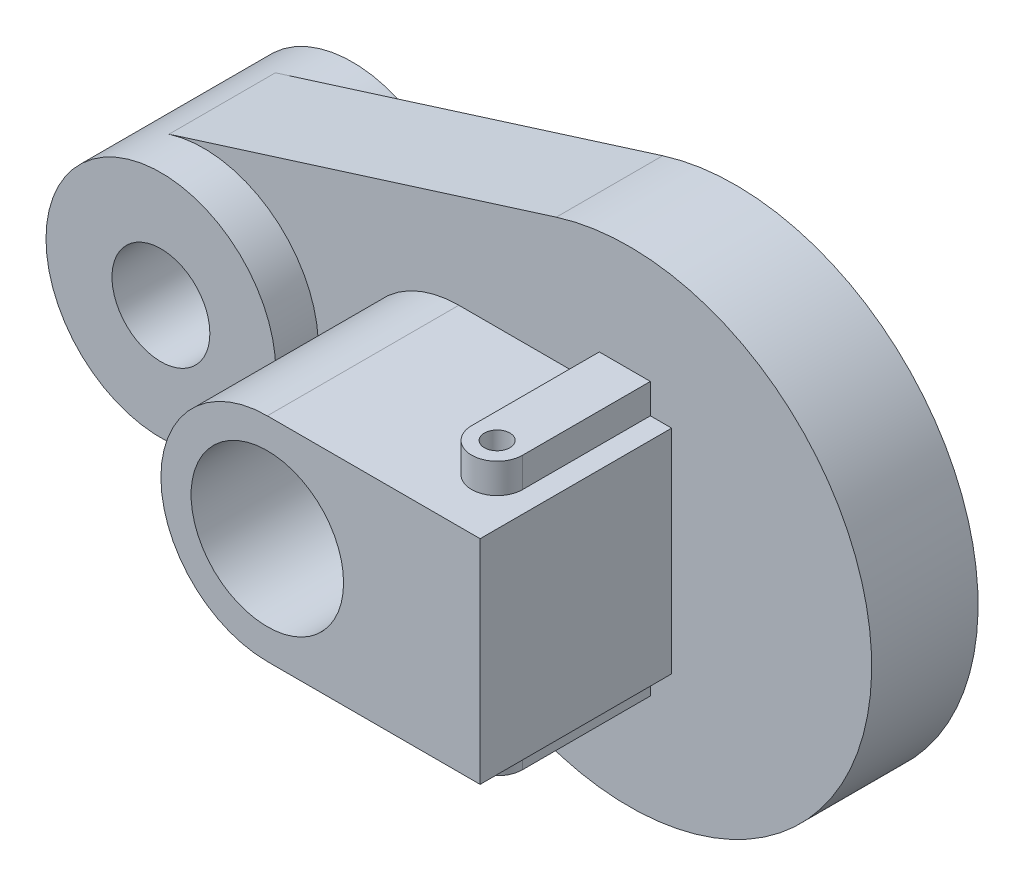
ISO-10303-21;
HEADER;
FILE_DESCRIPTION(('STEP AP214'),'2;1');
FILE_NAME('part.step','',(''),(''),'','','');
FILE_SCHEMA(('AUTOMOTIVE_DESIGN { 1 0 10303 214 1 1 1 1 }'));
ENDSEC;
DATA;
#1=APPLICATION_CONTEXT('core data for automotive mechanical design processes');
#2=APPLICATION_PROTOCOL_DEFINITION('international standard','automotive_design',2000,#1);
#3=PRODUCT_CONTEXT('',#1,'mechanical');
#4=PRODUCT('Part','Part','',(#3));
#5=PRODUCT_RELATED_PRODUCT_CATEGORY('part','',(#4));
#6=PRODUCT_DEFINITION_FORMATION('','',#4);
#7=PRODUCT_DEFINITION_CONTEXT('part definition',#1,'design');
#8=PRODUCT_DEFINITION('design','',#6,#7);
#9=PRODUCT_DEFINITION_SHAPE('','',#8);
#10=(LENGTH_UNIT() NAMED_UNIT(*) SI_UNIT(.MILLI.,.METRE.));
#11=(NAMED_UNIT(*) PLANE_ANGLE_UNIT() SI_UNIT($,.RADIAN.));
#12=(NAMED_UNIT(*) SI_UNIT($,.STERADIAN.) SOLID_ANGLE_UNIT());
#13=UNCERTAINTY_MEASURE_WITH_UNIT(LENGTH_MEASURE(1.E-05),#10,'distance_accuracy_value','');
#14=(GEOMETRIC_REPRESENTATION_CONTEXT(3) GLOBAL_UNCERTAINTY_ASSIGNED_CONTEXT((#13)) GLOBAL_UNIT_ASSIGNED_CONTEXT((#10,
#11,#12)) REPRESENTATION_CONTEXT('',''));
#15=CARTESIAN_POINT('',(0.,0.,0.));
#16=DIRECTION('',(0.,0.,1.));
#17=DIRECTION('',(1.,0.,0.));
#18=AXIS2_PLACEMENT_3D('',#15,#16,#17);
#19=CARTESIAN_POINT('',(0.,0.,25.));
#20=DIRECTION('',(0.,0.,1.));
#21=DIRECTION('',(1.,0.,0.));
#22=AXIS2_PLACEMENT_3D('',#19,#20,#21);
#23=PLANE('',#22);
#24=CARTESIAN_POINT('',(-99.9999999999951,0.,25.));
#25=DIRECTION('',(0.,0.,1.));
#26=DIRECTION('',(1.,0.,0.));
#27=AXIS2_PLACEMENT_3D('',#24,#25,#26);
#28=CIRCLE('',#27,26.9999999999953);
#29=CARTESIAN_POINT('',(-108.050824082347,-25.7717719917503,25.));
#30=VERTEX_POINT('',#29);
#31=CARTESIAN_POINT('',(-108.100000000003,25.7563584382502,25.));
#32=VERTEX_POINT('',#31);
#33=EDGE_CURVE('E11',#30,#32,#28,.T.);
#34=ORIENTED_EDGE('',*,*,#33,.F.);
#35=DIRECTION('',(0.954225072155131,-0.299089471012498,0.));
#36=VECTOR('',#35,1.);
#37=CARTESIAN_POINT('',(-17.0208632069058,-54.3039324211904,25.));
#38=LINE('',#37,#36);
#39=CARTESIAN_POINT('',(-20.0941700871881,-53.3406442453654,25.));
#40=VERTEX_POINT('',#39);
#41=EDGE_CURVE('E329',#30,#40,#38,.T.);
#42=ORIENTED_EDGE('',*,*,#41,.T.);
#43=CARTESIAN_POINT('',(0.,0.,25.));
#44=DIRECTION('',(0.,0.,1.));
#45=DIRECTION('',(1.,0.,0.));
#46=AXIS2_PLACEMENT_3D('',#43,#44,#45);
#47=CIRCLE('',#46,57.0000000000306);
#48=CARTESIAN_POINT('',(-17.1000000000286,54.3745344807889,25.));
#49=VERTEX_POINT('',#48);
#50=EDGE_CURVE('E338',#40,#49,#47,.T.);
#51=ORIENTED_EDGE('',*,*,#50,.T.);
#52=DIRECTION('',(0.953939201416839,0.30000000000034,0.));
#53=VECTOR('',#52,1.);
#54=CARTESIAN_POINT('',(-17.1000000000286,54.3745344807889,25.));
#55=LINE('',#54,#53);
#56=EDGE_CURVE('E343',#32,#49,#55,.T.);
#57=ORIENTED_EDGE('',*,*,#56,.F.);
#58=EDGE_LOOP('',(#34,#42,#51,#57));
#59=FACE_BOUND('',#58,.T.);
#60=DIRECTION('',(-1.,0.,0.));
#61=VECTOR('',#60,1.);
#62=CARTESIAN_POINT('',(-40.,25.,25.));
#63=LINE('',#62,#61);
#64=CARTESIAN_POINT('',(-6.99999999999999,25.,25.));
#65=VERTEX_POINT('',#64);
#66=CARTESIAN_POINT('',(-40.,25.,25.));
#67=VERTEX_POINT('',#66);
#68=EDGE_CURVE('E257',#65,#67,#63,.T.);
#69=ORIENTED_EDGE('',*,*,#68,.F.);
#70=DIRECTION('',(0.,-1.,0.));
#71=VECTOR('',#70,1.);
#72=CARTESIAN_POINT('',(-6.99999999999999,32.,25.));
#73=LINE('',#72,#71);
#74=CARTESIAN_POINT('',(-6.99999999999999,32.,25.));
#75=VERTEX_POINT('',#74);
#76=EDGE_CURVE('E63',#75,#65,#73,.T.);
#77=ORIENTED_EDGE('',*,*,#76,.F.);
#78=DIRECTION('',(-1.,0.,0.));
#79=VECTOR('',#78,1.);
#80=CARTESIAN_POINT('',(-6.99999999999999,32.,25.));
#81=LINE('',#80,#79);
#82=CARTESIAN_POINT('',(5.00000000000001,32.,25.));
#83=VERTEX_POINT('',#82);
#84=EDGE_CURVE('E68',#83,#75,#81,.T.);
#85=ORIENTED_EDGE('',*,*,#84,.F.);
#86=DIRECTION('',(0.,-1.,0.));
#87=VECTOR('',#86,1.);
#88=CARTESIAN_POINT('',(5.00000000000001,32.,25.));
#89=LINE('',#88,#87);
#90=CARTESIAN_POINT('',(5.00000000000001,25.,25.));
#91=VERTEX_POINT('',#90);
#92=EDGE_CURVE('E186',#83,#91,#89,.T.);
#93=ORIENTED_EDGE('',*,*,#92,.T.);
#94=CARTESIAN_POINT('',(10.,25.,25.));
#95=VERTEX_POINT('',#94);
#96=EDGE_CURVE('E244',#95,#91,#63,.T.);
#97=ORIENTED_EDGE('',*,*,#96,.F.);
#98=DIRECTION('',(0.,1.,0.));
#99=VECTOR('',#98,1.);
#100=CARTESIAN_POINT('',(10.,25.,25.));
#101=LINE('',#100,#99);
#102=CARTESIAN_POINT('',(10.,-25.,25.));
#103=VERTEX_POINT('',#102);
#104=EDGE_CURVE('E256',#103,#95,#101,.T.);
#105=ORIENTED_EDGE('',*,*,#104,.F.);
#106=DIRECTION('',(1.,0.,0.));
#107=VECTOR('',#106,1.);
#108=CARTESIAN_POINT('',(10.,-25.,25.));
#109=LINE('',#108,#107);
#110=CARTESIAN_POINT('',(5.00000000000001,-25.,25.));
#111=VERTEX_POINT('',#110);
#112=EDGE_CURVE('E251',#111,#103,#109,.T.);
#113=ORIENTED_EDGE('',*,*,#112,.F.);
#114=DIRECTION('',(0.,1.,0.));
#115=VECTOR('',#114,1.);
#116=CARTESIAN_POINT('',(5.00000000000001,-32.,25.));
#117=LINE('',#116,#115);
#118=CARTESIAN_POINT('',(5.00000000000001,-32.,25.));
#119=VERTEX_POINT('',#118);
#120=EDGE_CURVE('E233',#119,#111,#117,.T.);
#121=ORIENTED_EDGE('',*,*,#120,.F.);
#122=DIRECTION('',(1.,0.,0.));
#123=VECTOR('',#122,1.);
#124=CARTESIAN_POINT('',(-6.99999999999999,-32.,25.));
#125=LINE('',#124,#123);
#126=CARTESIAN_POINT('',(-6.99999999999999,-32.,25.));
#127=VERTEX_POINT('',#126);
#128=EDGE_CURVE('E203',#127,#119,#125,.T.);
#129=ORIENTED_EDGE('',*,*,#128,.F.);
#130=DIRECTION('',(0.,1.,0.));
#131=VECTOR('',#130,1.);
#132=CARTESIAN_POINT('',(-6.99999999999999,-32.,25.));
#133=LINE('',#132,#131);
#134=CARTESIAN_POINT('',(-6.99999999999999,-25.,25.));
#135=VERTEX_POINT('',#134);
#136=EDGE_CURVE('E212',#127,#135,#133,.T.);
#137=ORIENTED_EDGE('',*,*,#136,.T.);
#138=CARTESIAN_POINT('',(-40.,-25.,25.));
#139=VERTEX_POINT('',#138);
#140=EDGE_CURVE('E253',#139,#135,#109,.T.);
#141=ORIENTED_EDGE('',*,*,#140,.F.);
#142=CARTESIAN_POINT('',(-40.,0.,25.));
#143=DIRECTION('',(0.,0.,1.));
#144=DIRECTION('',(1.,0.,0.));
#145=AXIS2_PLACEMENT_3D('',#142,#143,#144);
#146=CIRCLE('',#145,25.);
#147=EDGE_CURVE('E238',#67,#139,#146,.T.);
#148=ORIENTED_EDGE('',*,*,#147,.F.);
#149=EDGE_LOOP('',(#69,#77,#85,#93,#97,#105,#113,#121,#129,#137,#141,#148));
#150=FACE_BOUND('',#149,.T.);
#151=ADVANCED_FACE('F50',(#59,#150),#23,.T.);
#152=CARTESIAN_POINT('',(-40.,25.,70.));
#153=DIRECTION('',(0.,-1.,0.));
#154=DIRECTION('',(0.,0.,-1.));
#155=AXIS2_PLACEMENT_3D('',#152,#153,#154);
#156=PLANE('',#155);
#157=DIRECTION('',(0.,0.,1.));
#158=VECTOR('',#157,1.);
#159=CARTESIAN_POINT('',(-6.99999999999999,25.,55.));
#160=LINE('',#159,#158);
#161=CARTESIAN_POINT('',(-6.99999999999999,25.,55.));
#162=VERTEX_POINT('',#161);
#163=EDGE_CURVE('E177',#65,#162,#160,.T.);
#164=ORIENTED_EDGE('',*,*,#163,.F.);
#165=ORIENTED_EDGE('',*,*,#68,.T.);
#166=DIRECTION('',(0.,0.,-1.));
#167=VECTOR('',#166,1.);
#168=CARTESIAN_POINT('',(-40.,25.,70.));
#169=LINE('',#168,#167);
#170=CARTESIAN_POINT('',(-40.,25.,70.));
#171=VERTEX_POINT('',#170);
#172=EDGE_CURVE('E252',#171,#67,#169,.T.);
#173=ORIENTED_EDGE('',*,*,#172,.F.);
#174=DIRECTION('',(-1.,0.,0.));
#175=VECTOR('',#174,1.);
#176=CARTESIAN_POINT('',(-40.,25.,70.));
#177=LINE('',#176,#175);
#178=CARTESIAN_POINT('',(10.,25.,70.));
#179=VERTEX_POINT('',#178);
#180=EDGE_CURVE('E248',#179,#171,#177,.T.);
#181=ORIENTED_EDGE('',*,*,#180,.F.);
#182=DIRECTION('',(0.,0.,-1.));
#183=VECTOR('',#182,1.);
#184=CARTESIAN_POINT('',(10.,25.,70.));
#185=LINE('',#184,#183);
#186=EDGE_CURVE('E263',#179,#95,#185,.T.);
#187=ORIENTED_EDGE('',*,*,#186,.T.);
#188=ORIENTED_EDGE('',*,*,#96,.T.);
#189=DIRECTION('',(0.,0.,-1.));
#190=VECTOR('',#189,1.);
#191=CARTESIAN_POINT('',(5.00000000000001,25.,25.));
#192=LINE('',#191,#190);
#193=CARTESIAN_POINT('',(5.00000000000001,25.,55.));
#194=VERTEX_POINT('',#193);
#195=EDGE_CURVE('E200',#194,#91,#192,.T.);
#196=ORIENTED_EDGE('',*,*,#195,.F.);
#197=CARTESIAN_POINT('',(-0.999999999999991,25.,55.));
#198=DIRECTION('',(0.,1.,0.));
#199=DIRECTION('',(0.,0.,1.));
#200=AXIS2_PLACEMENT_3D('',#197,#198,#199);
#201=CIRCLE('',#200,6.);
#202=EDGE_CURVE('E193',#162,#194,#201,.T.);
#203=ORIENTED_EDGE('',*,*,#202,.F.);
#204=EDGE_LOOP('',(#164,#165,#173,#181,#187,#188,#196,#203));
#205=FACE_BOUND('',#204,.T.);
#206=ADVANCED_FACE('F374',(#205),#156,.F.);
#207=CARTESIAN_POINT('',(10.,-25.,70.));
#208=DIRECTION('',(0.,1.,0.));
#209=DIRECTION('',(0.,0.,1.));
#210=AXIS2_PLACEMENT_3D('',#207,#208,#209);
#211=PLANE('',#210);
#212=DIRECTION('',(0.,0.,1.));
#213=VECTOR('',#212,1.);
#214=CARTESIAN_POINT('',(5.00000000000001,-25.,25.));
#215=LINE('',#214,#213);
#216=CARTESIAN_POINT('',(5.00000000000001,-25.,55.));
#217=VERTEX_POINT('',#216);
#218=EDGE_CURVE('E205',#111,#217,#215,.T.);
#219=ORIENTED_EDGE('',*,*,#218,.F.);
#220=ORIENTED_EDGE('',*,*,#112,.T.);
#221=DIRECTION('',(0.,0.,-1.));
#222=VECTOR('',#221,1.);
#223=CARTESIAN_POINT('',(10.,-25.,70.));
#224=LINE('',#223,#222);
#225=CARTESIAN_POINT('',(10.,-25.,70.));
#226=VERTEX_POINT('',#225);
#227=EDGE_CURVE('E269',#226,#103,#224,.T.);
#228=ORIENTED_EDGE('',*,*,#227,.F.);
#229=DIRECTION('',(1.,0.,0.));
#230=VECTOR('',#229,1.);
#231=CARTESIAN_POINT('',(10.,-25.,70.));
#232=LINE('',#231,#230);
#233=CARTESIAN_POINT('',(-40.,-25.,70.));
#234=VERTEX_POINT('',#233);
#235=EDGE_CURVE('E242',#234,#226,#232,.T.);
#236=ORIENTED_EDGE('',*,*,#235,.F.);
#237=DIRECTION('',(0.,0.,-1.));
#238=VECTOR('',#237,1.);
#239=CARTESIAN_POINT('',(-40.,-25.,70.));
#240=LINE('',#239,#238);
#241=EDGE_CURVE('E268',#234,#139,#240,.T.);
#242=ORIENTED_EDGE('',*,*,#241,.T.);
#243=ORIENTED_EDGE('',*,*,#140,.T.);
#244=DIRECTION('',(0.,0.,-1.));
#245=VECTOR('',#244,1.);
#246=CARTESIAN_POINT('',(-6.99999999999999,-25.,55.));
#247=LINE('',#246,#245);
#248=CARTESIAN_POINT('',(-6.99999999999999,-25.,55.));
#249=VERTEX_POINT('',#248);
#250=EDGE_CURVE('E206',#249,#135,#247,.T.);
#251=ORIENTED_EDGE('',*,*,#250,.F.);
#252=CARTESIAN_POINT('',(-0.999999999999989,-25.,55.));
#253=DIRECTION('',(0.,-1.,0.));
#254=DIRECTION('',(0.,0.,-1.));
#255=AXIS2_PLACEMENT_3D('',#252,#253,#254);
#256=CIRCLE('',#255,6.);
#257=EDGE_CURVE('E217',#217,#249,#256,.T.);
#258=ORIENTED_EDGE('',*,*,#257,.F.);
#259=EDGE_LOOP('',(#219,#220,#228,#236,#242,#243,#251,#258));
#260=FACE_BOUND('',#259,.T.);
#261=ADVANCED_FACE('F367',(#260),#211,.F.);
#262=CARTESIAN_POINT('',(0.,0.,0.));
#263=DIRECTION('',(0.,0.,1.));
#264=DIRECTION('',(1.,0.,0.));
#265=AXIS2_PLACEMENT_3D('',#262,#263,#264);
#266=PLANE('',#265);
#267=CARTESIAN_POINT('',(-99.9999999999951,0.,0.));
#268=DIRECTION('',(0.,0.,-1.));
#269=DIRECTION('',(-1.,0.,0.));
#270=AXIS2_PLACEMENT_3D('',#267,#268,#269);
#271=CIRCLE('',#270,27.0000000000047);
#272=CARTESIAN_POINT('',(-108.100000000006,25.7563584382591,0.));
#273=VERTEX_POINT('',#272);
#274=CARTESIAN_POINT('',(-108.050824073021,-25.7717719946737,0.));
#275=VERTEX_POINT('',#274);
#276=EDGE_CURVE('E280',#273,#275,#271,.T.);
#277=ORIENTED_EDGE('',*,*,#276,.F.);
#278=DIRECTION('',(0.953939201416839,0.30000000000034,0.));
#279=VECTOR('',#278,1.);
#280=CARTESIAN_POINT('',(-17.1000000000286,54.3745344807889,0.));
#281=LINE('',#280,#279);
#282=CARTESIAN_POINT('',(-17.1000000000286,54.3745344807889,0.));
#283=VERTEX_POINT('',#282);
#284=EDGE_CURVE('E342',#273,#283,#281,.T.);
#285=ORIENTED_EDGE('',*,*,#284,.T.);
#286=CARTESIAN_POINT('',(0.,0.,0.));
#287=DIRECTION('',(0.,0.,1.));
#288=DIRECTION('',(1.,0.,0.));
#289=AXIS2_PLACEMENT_3D('',#286,#287,#288);
#290=CIRCLE('',#289,57.0000000000306);
#291=CARTESIAN_POINT('',(-20.0941700871881,-53.3406442453654,0.));
#292=VERTEX_POINT('',#291);
#293=EDGE_CURVE('E344',#292,#283,#290,.T.);
#294=ORIENTED_EDGE('',*,*,#293,.F.);
#295=DIRECTION('',(0.954225072155131,-0.299089471012498,0.));
#296=VECTOR('',#295,1.);
#297=CARTESIAN_POINT('',(-17.0208632069058,-54.3039324211904,0.));
#298=LINE('',#297,#296);
#299=EDGE_CURVE('E300',#275,#292,#298,.T.);
#300=ORIENTED_EDGE('',*,*,#299,.F.);
#301=EDGE_LOOP('',(#277,#285,#294,#300));
#302=FACE_BOUND('',#301,.T.);
#303=ADVANCED_FACE('F370',(#302),#266,.F.);
#304=CARTESIAN_POINT('',(-17.1000000000286,54.3745344807889,25.));
#305=DIRECTION('',(-0.30000000000034,0.953939201416839,0.));
#306=DIRECTION('',(-0.953939201416839,-0.30000000000034,0.));
#307=AXIS2_PLACEMENT_3D('',#304,#305,#306);
#308=PLANE('',#307);
#309=ORIENTED_EDGE('',*,*,#284,.F.);
#310=DIRECTION('',(0.,0.,-1.));
#311=VECTOR('',#310,1.);
#312=CARTESIAN_POINT('',(-108.100000000004,25.7563584382527,25.));
#313=LINE('',#312,#311);
#314=EDGE_CURVE('E57',#32,#273,#313,.T.);
#315=ORIENTED_EDGE('',*,*,#314,.F.);
#316=ORIENTED_EDGE('',*,*,#56,.T.);
#317=DIRECTION('',(0.,0.,-1.));
#318=VECTOR('',#317,1.);
#319=CARTESIAN_POINT('',(-17.1000000000286,54.3745344807889,25.));
#320=LINE('',#319,#318);
#321=EDGE_CURVE('E336',#49,#283,#320,.T.);
#322=ORIENTED_EDGE('',*,*,#321,.T.);
#323=EDGE_LOOP('',(#309,#315,#316,#322));
#324=FACE_BOUND('',#323,.T.);
#325=ADVANCED_FACE('F47',(#324),#308,.T.);
#326=CARTESIAN_POINT('',(-99.9999999999951,0.,25.));
#327=DIRECTION('',(0.,0.,-1.));
#328=DIRECTION('',(-1.,0.,0.));
#329=AXIS2_PLACEMENT_3D('',#326,#327,#328);
#330=CYLINDRICAL_SURFACE('',#329,26.999999999998);
#331=ORIENTED_EDGE('',*,*,#314,.T.);
#332=ORIENTED_EDGE('',*,*,#276,.T.);
#333=CARTESIAN_POINT('',(-108.100000000004,-25.7563584382527,0.));
#334=DIRECTION('',(0.95422507215511,-0.299089471012563,0.));
#335=VECTOR('',#334,1.);
#336=LINE('',#333,#335);
#337=CARTESIAN_POINT('',(-108.100000000004,-25.7563584382527,0.));
#338=VERTEX_POINT('',#337);
#339=EDGE_CURVE('E292',#338,#275,#336,.T.);
#340=ORIENTED_EDGE('',*,*,#339,.F.);
#341=DIRECTION('',(0.,0.,-1.));
#342=VECTOR('',#341,1.);
#343=CARTESIAN_POINT('',(-108.100000000004,-25.7563584382527,25.));
#344=LINE('',#343,#342);
#345=CARTESIAN_POINT('',(-108.100000000004,-25.7563584382527,25.));
#346=VERTEX_POINT('',#345);
#347=EDGE_CURVE('E318',#346,#338,#344,.T.);
#348=ORIENTED_EDGE('',*,*,#347,.F.);
#349=CARTESIAN_POINT('',(-99.9999999999951,0.,25.));
#350=DIRECTION('',(0.,0.,1.));
#351=DIRECTION('',(-0.30000000000034,-0.953939201416839,0.));
#352=AXIS2_PLACEMENT_3D('',#349,#350,#351);
#353=CIRCLE('',#352,26.999999999998);
#354=EDGE_CURVE('E347',#346,#30,#353,.T.);
#355=ORIENTED_EDGE('',*,*,#354,.T.);
#356=ORIENTED_EDGE('',*,*,#33,.T.);
#357=EDGE_LOOP('',(#331,#332,#340,#348,#355,#356));
#358=FACE_BOUND('',#357,.T.);
#359=CARTESIAN_POINT('',(-99.9999999999951,0.,35.));
#360=DIRECTION('',(0.,0.,1.));
#361=DIRECTION('',(1.,0.,0.));
#362=AXIS2_PLACEMENT_3D('',#359,#360,#361);
#363=CIRCLE('',#362,26.9999999999953);
#364=CARTESIAN_POINT('',(-72.9999999999998,0.,35.));
#365=VERTEX_POINT('',#364);
#366=EDGE_CURVE('E276',#365,#365,#363,.T.);
#367=ORIENTED_EDGE('',*,*,#366,.F.);
#368=EDGE_LOOP('',(#367));
#369=FACE_BOUND('',#368,.T.);
#370=CARTESIAN_POINT('',(-99.9999999999951,0.,-10.));
#371=DIRECTION('',(0.,0.,-1.));
#372=DIRECTION('',(-1.,0.,0.));
#373=AXIS2_PLACEMENT_3D('',#370,#371,#372);
#374=CIRCLE('',#373,27.0000000000047);
#375=CARTESIAN_POINT('',(-127.,0.,-10.));
#376=VERTEX_POINT('',#375);
#377=EDGE_CURVE('E274',#376,#376,#374,.T.);
#378=ORIENTED_EDGE('',*,*,#377,.F.);
#379=EDGE_LOOP('',(#378));
#380=FACE_BOUND('',#379,.T.);
#381=ADVANCED_FACE('F307',(#358,#369,#380),#330,.T.);
#382=CARTESIAN_POINT('',(-17.0208632069058,-54.3039324211904,25.));
#383=DIRECTION('',(0.299089471012498,0.954225072155131,0.));
#384=DIRECTION('',(-0.954225072155131,0.299089471012498,0.));
#385=AXIS2_PLACEMENT_3D('',#382,#383,#384);
#386=PLANE('',#385);
#387=ORIENTED_EDGE('',*,*,#339,.T.);
#388=ORIENTED_EDGE('',*,*,#299,.T.);
#389=DIRECTION('',(0.,0.,-1.));
#390=VECTOR('',#389,1.);
#391=CARTESIAN_POINT('',(-20.0941700871881,-53.3406442453654,25.));
#392=LINE('',#391,#390);
#393=EDGE_CURVE('E330',#40,#292,#392,.T.);
#394=ORIENTED_EDGE('',*,*,#393,.F.);
#395=ORIENTED_EDGE('',*,*,#41,.F.);
#396=ORIENTED_EDGE('',*,*,#354,.F.);
#397=ORIENTED_EDGE('',*,*,#347,.T.);
#398=EDGE_LOOP('',(#387,#388,#394,#395,#396,#397));
#399=FACE_BOUND('',#398,.T.);
#400=ADVANCED_FACE('F299',(#399),#386,.F.);
#401=CARTESIAN_POINT('',(0.,0.,25.));
#402=DIRECTION('',(0.,0.,-1.));
#403=DIRECTION('',(-1.,0.,0.));
#404=AXIS2_PLACEMENT_3D('',#401,#402,#403);
#405=CYLINDRICAL_SURFACE('',#404,57.0000000000306);
#406=ORIENTED_EDGE('',*,*,#293,.T.);
#407=ORIENTED_EDGE('',*,*,#321,.F.);
#408=ORIENTED_EDGE('',*,*,#50,.F.);
#409=ORIENTED_EDGE('',*,*,#393,.T.);
#410=EDGE_LOOP('',(#406,#407,#408,#409));
#411=FACE_BOUND('',#410,.T.);
#412=ADVANCED_FACE('F308',(#411),#405,.T.);
#413=CARTESIAN_POINT('',(-99.9999999999951,0.,35.));
#414=DIRECTION('',(0.,0.,1.));
#415=DIRECTION('',(1.,0.,0.));
#416=AXIS2_PLACEMENT_3D('',#413,#414,#415);
#417=PLANE('',#416);
#418=CARTESIAN_POINT('',(-99.9999999999951,0.,35.));
#419=DIRECTION('',(0.,0.,1.));
#420=DIRECTION('',(1.,0.,0.));
#421=AXIS2_PLACEMENT_3D('',#418,#419,#420);
#422=CIRCLE('',#421,11.4999999999953);
#423=CARTESIAN_POINT('',(-88.4999999999998,0.,35.));
#424=VERTEX_POINT('',#423);
#425=EDGE_CURVE('E272',#424,#424,#422,.T.);
#426=ORIENTED_EDGE('',*,*,#425,.F.);
#427=EDGE_LOOP('',(#426));
#428=FACE_BOUND('',#427,.T.);
#429=ORIENTED_EDGE('',*,*,#366,.T.);
#430=EDGE_LOOP('',(#429));
#431=FACE_BOUND('',#430,.T.);
#432=ADVANCED_FACE('F390',(#428,#431),#417,.T.);
#433=CARTESIAN_POINT('',(-99.9999999999951,0.,-10.));
#434=DIRECTION('',(0.,0.,-1.));
#435=DIRECTION('',(-1.,0.,0.));
#436=AXIS2_PLACEMENT_3D('',#433,#434,#435);
#437=PLANE('',#436);
#438=CARTESIAN_POINT('',(-99.9999999999951,0.,-10.));
#439=DIRECTION('',(0.,0.,-1.));
#440=DIRECTION('',(-1.,0.,0.));
#441=AXIS2_PLACEMENT_3D('',#438,#439,#440);
#442=CIRCLE('',#441,11.4999999999953);
#443=CARTESIAN_POINT('',(-111.49999999999,0.,-10.));
#444=VERTEX_POINT('',#443);
#445=EDGE_CURVE('E51',#444,#444,#442,.T.);
#446=ORIENTED_EDGE('',*,*,#445,.F.);
#447=EDGE_LOOP('',(#446));
#448=FACE_BOUND('',#447,.T.);
#449=ORIENTED_EDGE('',*,*,#377,.T.);
#450=EDGE_LOOP('',(#449));
#451=FACE_BOUND('',#450,.T.);
#452=ADVANCED_FACE('F391',(#448,#451),#437,.T.);
#453=CARTESIAN_POINT('',(-99.9999999999951,0.,-15.));
#454=DIRECTION('',(0.,0.,1.));
#455=DIRECTION('',(1.,0.,0.));
#456=AXIS2_PLACEMENT_3D('',#453,#454,#455);
#457=CYLINDRICAL_SURFACE('',#456,11.4999999999953);
#458=ORIENTED_EDGE('',*,*,#445,.T.);
#459=EDGE_LOOP('',(#458));
#460=FACE_BOUND('',#459,.T.);
#461=ORIENTED_EDGE('',*,*,#425,.T.);
#462=EDGE_LOOP('',(#461));
#463=FACE_BOUND('',#462,.T.);
#464=ADVANCED_FACE('F394',(#460,#463),#457,.F.);
#465=CARTESIAN_POINT('',(-40.,0.,70.));
#466=DIRECTION('',(0.,0.,-1.));
#467=DIRECTION('',(-1.,0.,0.));
#468=AXIS2_PLACEMENT_3D('',#465,#466,#467);
#469=CYLINDRICAL_SURFACE('',#468,25.);
#470=ORIENTED_EDGE('',*,*,#147,.T.);
#471=ORIENTED_EDGE('',*,*,#241,.F.);
#472=CARTESIAN_POINT('',(-40.,0.,70.));
#473=DIRECTION('',(0.,0.,1.));
#474=DIRECTION('',(1.,0.,0.));
#475=AXIS2_PLACEMENT_3D('',#472,#473,#474);
#476=CIRCLE('',#475,25.);
#477=EDGE_CURVE('E241',#171,#234,#476,.T.);
#478=ORIENTED_EDGE('',*,*,#477,.F.);
#479=ORIENTED_EDGE('',*,*,#172,.T.);
#480=EDGE_LOOP('',(#470,#471,#478,#479));
#481=FACE_BOUND('',#480,.T.);
#482=ADVANCED_FACE('F398',(#481),#469,.T.);
#483=CARTESIAN_POINT('',(10.,25.,70.));
#484=DIRECTION('',(-1.,0.,0.));
#485=DIRECTION('',(0.,0.,1.));
#486=AXIS2_PLACEMENT_3D('',#483,#484,#485);
#487=PLANE('',#486);
#488=ORIENTED_EDGE('',*,*,#104,.T.);
#489=ORIENTED_EDGE('',*,*,#186,.F.);
#490=DIRECTION('',(0.,1.,0.));
#491=VECTOR('',#490,1.);
#492=CARTESIAN_POINT('',(10.,25.,70.));
#493=LINE('',#492,#491);
#494=EDGE_CURVE('E250',#226,#179,#493,.T.);
#495=ORIENTED_EDGE('',*,*,#494,.F.);
#496=ORIENTED_EDGE('',*,*,#227,.T.);
#497=EDGE_LOOP('',(#488,#489,#495,#496));
#498=FACE_BOUND('',#497,.T.);
#499=ADVANCED_FACE('F405',(#498),#487,.F.);
#500=CARTESIAN_POINT('',(-40.,0.,70.));
#501=DIRECTION('',(0.,0.,1.));
#502=DIRECTION('',(1.,0.,0.));
#503=AXIS2_PLACEMENT_3D('',#500,#501,#502);
#504=PLANE('',#503);
#505=CARTESIAN_POINT('',(-40.,0.,70.));
#506=DIRECTION('',(0.,0.,1.));
#507=DIRECTION('',(1.,0.,0.));
#508=AXIS2_PLACEMENT_3D('',#505,#506,#507);
#509=CIRCLE('',#508,17.9127372990422);
#510=CARTESIAN_POINT('',(-22.0872627009578,0.,70.));
#511=VERTEX_POINT('',#510);
#512=EDGE_CURVE('E234',#511,#511,#509,.T.);
#513=ORIENTED_EDGE('',*,*,#512,.F.);
#514=EDGE_LOOP('',(#513));
#515=FACE_BOUND('',#514,.T.);
#516=ORIENTED_EDGE('',*,*,#477,.T.);
#517=ORIENTED_EDGE('',*,*,#235,.T.);
#518=ORIENTED_EDGE('',*,*,#494,.T.);
#519=ORIENTED_EDGE('',*,*,#180,.T.);
#520=EDGE_LOOP('',(#516,#517,#518,#519));
#521=FACE_BOUND('',#520,.T.);
#522=ADVANCED_FACE('F409',(#515,#521),#504,.T.);
#523=CARTESIAN_POINT('',(-40.,0.,25.));
#524=DIRECTION('',(0.,0.,1.));
#525=DIRECTION('',(1.,0.,0.));
#526=AXIS2_PLACEMENT_3D('',#523,#524,#525);
#527=CYLINDRICAL_SURFACE('',#526,17.9127372990422);
#528=CARTESIAN_POINT('',(-40.,0.,25.));
#529=DIRECTION('',(0.,0.,1.));
#530=DIRECTION('',(1.,0.,0.));
#531=AXIS2_PLACEMENT_3D('',#528,#529,#530);
#532=CIRCLE('',#531,17.9127372990422);
#533=CARTESIAN_POINT('',(-22.0872627009578,0.,25.));
#534=VERTEX_POINT('',#533);
#535=EDGE_CURVE('E232',#534,#534,#532,.T.);
#536=CARTESIAN_POINT('',(-22.0872627009578,0.,25.));
#537=CARTESIAN_POINT('',(-22.0872627009578,0.,25.46875));
#538=CARTESIAN_POINT('',(-22.0872627009578,0.,25.9375));
#539=CARTESIAN_POINT('',(-22.0872627009578,0.,26.875));
#540=CARTESIAN_POINT('',(-22.0872627009578,0.,27.34375));
#541=CARTESIAN_POINT('',(-22.0872627009578,0.,28.28125));
#542=CARTESIAN_POINT('',(-22.0872627009578,0.,28.75));
#543=CARTESIAN_POINT('',(-22.0872627009578,0.,29.6875));
#544=CARTESIAN_POINT('',(-22.0872627009578,0.,30.15625));
#545=CARTESIAN_POINT('',(-22.0872627009578,0.,31.09375));
#546=CARTESIAN_POINT('',(-22.0872627009578,0.,31.5625));
#547=CARTESIAN_POINT('',(-22.0872627009578,0.,32.5));
#548=CARTESIAN_POINT('',(-22.0872627009578,0.,32.96875));
#549=CARTESIAN_POINT('',(-22.0872627009578,0.,33.90625));
#550=CARTESIAN_POINT('',(-22.0872627009578,0.,34.375));
#551=CARTESIAN_POINT('',(-22.0872627009578,0.,35.3125));
#552=CARTESIAN_POINT('',(-22.0872627009578,0.,35.78125));
#553=CARTESIAN_POINT('',(-22.0872627009578,0.,36.71875));
#554=CARTESIAN_POINT('',(-22.0872627009578,0.,37.1875));
#555=CARTESIAN_POINT('',(-22.0872627009578,0.,38.125));
#556=CARTESIAN_POINT('',(-22.0872627009578,0.,38.59375));
#557=CARTESIAN_POINT('',(-22.0872627009578,0.,39.53125));
#558=CARTESIAN_POINT('',(-22.0872627009578,0.,40.));
#559=CARTESIAN_POINT('',(-22.0872627009578,0.,40.9375));
#560=CARTESIAN_POINT('',(-22.0872627009578,0.,41.40625));
#561=CARTESIAN_POINT('',(-22.0872627009578,0.,42.34375));
#562=CARTESIAN_POINT('',(-22.0872627009578,0.,42.8125));
#563=CARTESIAN_POINT('',(-22.0872627009578,0.,43.75));
#564=CARTESIAN_POINT('',(-22.0872627009578,0.,44.21875));
#565=CARTESIAN_POINT('',(-22.0872627009578,0.,45.15625));
#566=CARTESIAN_POINT('',(-22.0872627009578,0.,45.625));
#567=CARTESIAN_POINT('',(-22.0872627009578,0.,46.5625));
#568=CARTESIAN_POINT('',(-22.0872627009578,0.,47.03125));
#569=CARTESIAN_POINT('',(-22.0872627009578,0.,47.96875));
#570=CARTESIAN_POINT('',(-22.0872627009578,0.,48.4375));
#571=CARTESIAN_POINT('',(-22.0872627009578,0.,49.375));
#572=CARTESIAN_POINT('',(-22.0872627009578,0.,49.84375));
#573=CARTESIAN_POINT('',(-22.0872627009578,0.,50.78125));
#574=CARTESIAN_POINT('',(-22.0872627009578,0.,51.25));
#575=CARTESIAN_POINT('',(-22.0872627009578,0.,52.1875));
#576=CARTESIAN_POINT('',(-22.0872627009578,0.,52.65625));
#577=CARTESIAN_POINT('',(-22.0872627009578,0.,53.59375));
#578=CARTESIAN_POINT('',(-22.0872627009578,0.,54.0625));
#579=CARTESIAN_POINT('',(-22.0872627009578,0.,55.));
#580=CARTESIAN_POINT('',(-22.0872627009578,0.,55.46875));
#581=CARTESIAN_POINT('',(-22.0872627009578,0.,56.40625));
#582=CARTESIAN_POINT('',(-22.0872627009578,0.,56.875));
#583=CARTESIAN_POINT('',(-22.0872627009578,0.,57.8125));
#584=CARTESIAN_POINT('',(-22.0872627009578,0.,58.28125));
#585=CARTESIAN_POINT('',(-22.0872627009578,0.,59.21875));
#586=CARTESIAN_POINT('',(-22.0872627009578,0.,59.6875));
#587=CARTESIAN_POINT('',(-22.0872627009578,0.,60.625));
#588=CARTESIAN_POINT('',(-22.0872627009578,0.,61.09375));
#589=CARTESIAN_POINT('',(-22.0872627009578,0.,62.03125));
#590=CARTESIAN_POINT('',(-22.0872627009578,0.,62.5));
#591=CARTESIAN_POINT('',(-22.0872627009578,0.,63.4375));
#592=CARTESIAN_POINT('',(-22.0872627009578,0.,63.90625));
#593=CARTESIAN_POINT('',(-22.0872627009578,0.,64.84375));
#594=CARTESIAN_POINT('',(-22.0872627009578,0.,65.3125));
#595=CARTESIAN_POINT('',(-22.0872627009578,0.,66.25));
#596=CARTESIAN_POINT('',(-22.0872627009578,0.,66.71875));
#597=CARTESIAN_POINT('',(-22.0872627009578,0.,67.65625));
#598=CARTESIAN_POINT('',(-22.0872627009578,0.,68.125));
#599=CARTESIAN_POINT('',(-22.0872627009578,0.,69.0625));
#600=CARTESIAN_POINT('',(-22.0872627009578,0.,69.53125));
#601=CARTESIAN_POINT('',(-22.0872627009578,0.,70.));
#602=B_SPLINE_CURVE_WITH_KNOTS('',3,(#536,#537,#538,#539,#540,#541,#542,#543,#544,#545,#546,
#547,#548,#549,#550,#551,#552,#553,#554,#555,#556,#557,#558,#559,#560,#561,#562,#563,#564,#565,
#566,#567,#568,#569,#570,#571,#572,#573,#574,#575,#576,#577,#578,#579,#580,#581,#582,#583,#584,
#585,#586,#587,#588,#589,#590,#591,#592,#593,#594,#595,#596,#597,#598,#599,#600,#601),
.UNSPECIFIED.,.F.,.F.,(4,2,2,2,2,2,2,2,2,2,2,2,2,2,2,2,2,2,2,2,2,2,2,2,2,2,2,2,2,2,2,2,4),(0.,
1.40625,2.8125,4.21875,5.625,7.03125,8.4375,9.84375,11.25,12.65625,14.0625,15.46875,16.875,
18.28125,19.6875,21.09375,22.5,23.90625,25.3125,26.71875,28.125,29.53125,30.9375,32.34375,33.75,
35.15625,36.5625,37.96875,39.375,40.78125,42.1875,43.59375,45.),.UNSPECIFIED.);
#603=EDGE_CURVE('BSEAM411',#534,#511,#602,.T.);
#604=ORIENTED_EDGE('',*,*,#535,.F.);
#605=ORIENTED_EDGE('',*,*,#512,.T.);
#606=ORIENTED_EDGE('',*,*,#603,.T.);
#607=ORIENTED_EDGE('',*,*,#603,.F.);
#608=EDGE_LOOP('',(#604,#606,#605,#607));
#609=FACE_BOUND('',#608,.T.);
#610=ADVANCED_FACE('F411',(#609),#527,.F.);
#611=CARTESIAN_POINT('',(-40.,0.,25.));
#612=DIRECTION('',(0.,0.,1.));
#613=DIRECTION('',(1.,0.,0.));
#614=AXIS2_PLACEMENT_3D('',#611,#612,#613);
#615=PLANE('',#614);
#616=ORIENTED_EDGE('',*,*,#535,.T.);
#617=EDGE_LOOP('',(#616));
#618=FACE_BOUND('',#617,.T.);
#619=ADVANCED_FACE('F414',(#618),#615,.T.);
#620=CARTESIAN_POINT('',(5.00000000000001,-32.,25.));
#621=DIRECTION('',(-1.,0.,0.));
#622=DIRECTION('',(0.,0.,1.));
#623=AXIS2_PLACEMENT_3D('',#620,#621,#622);
#624=PLANE('',#623);
#625=ORIENTED_EDGE('',*,*,#218,.T.);
#626=DIRECTION('',(0.,1.,0.));
#627=VECTOR('',#626,1.);
#628=CARTESIAN_POINT('',(5.00000000000001,-32.,55.));
#629=LINE('',#628,#627);
#630=CARTESIAN_POINT('',(5.00000000000001,-32.,55.));
#631=VERTEX_POINT('',#630);
#632=EDGE_CURVE('E226',#631,#217,#629,.T.);
#633=ORIENTED_EDGE('',*,*,#632,.F.);
#634=DIRECTION('',(0.,0.,1.));
#635=VECTOR('',#634,1.);
#636=CARTESIAN_POINT('',(5.00000000000001,-32.,25.));
#637=LINE('',#636,#635);
#638=EDGE_CURVE('E210',#119,#631,#637,.T.);
#639=ORIENTED_EDGE('',*,*,#638,.F.);
#640=ORIENTED_EDGE('',*,*,#120,.T.);
#641=EDGE_LOOP('',(#625,#633,#639,#640));
#642=FACE_BOUND('',#641,.T.);
#643=ADVANCED_FACE('F418',(#642),#624,.F.);
#644=CARTESIAN_POINT('',(-0.999999999999989,-32.,55.));
#645=DIRECTION('',(0.,1.,0.));
#646=DIRECTION('',(0.,0.,1.));
#647=AXIS2_PLACEMENT_3D('',#644,#645,#646);
#648=CYLINDRICAL_SURFACE('',#647,6.);
#649=ORIENTED_EDGE('',*,*,#257,.T.);
#650=DIRECTION('',(0.,1.,0.));
#651=VECTOR('',#650,1.);
#652=CARTESIAN_POINT('',(-6.99999999999999,-32.,55.));
#653=LINE('',#652,#651);
#654=CARTESIAN_POINT('',(-6.99999999999999,-32.,55.));
#655=VERTEX_POINT('',#654);
#656=EDGE_CURVE('E222',#655,#249,#653,.T.);
#657=ORIENTED_EDGE('',*,*,#656,.F.);
#658=CARTESIAN_POINT('',(-0.999999999999989,-32.,55.));
#659=DIRECTION('',(0.,-1.,0.));
#660=DIRECTION('',(0.,0.,-1.));
#661=AXIS2_PLACEMENT_3D('',#658,#659,#660);
#662=CIRCLE('',#661,6.);
#663=EDGE_CURVE('E208',#631,#655,#662,.T.);
#664=ORIENTED_EDGE('',*,*,#663,.F.);
#665=ORIENTED_EDGE('',*,*,#632,.T.);
#666=EDGE_LOOP('',(#649,#657,#664,#665));
#667=FACE_BOUND('',#666,.T.);
#668=ADVANCED_FACE('F421',(#667),#648,.T.);
#669=CARTESIAN_POINT('',(-6.99999999999999,-32.,55.));
#670=DIRECTION('',(1.,0.,0.));
#671=DIRECTION('',(0.,0.,-1.));
#672=AXIS2_PLACEMENT_3D('',#669,#670,#671);
#673=PLANE('',#672);
#674=ORIENTED_EDGE('',*,*,#250,.T.);
#675=ORIENTED_EDGE('',*,*,#136,.F.);
#676=DIRECTION('',(0.,0.,-1.));
#677=VECTOR('',#676,1.);
#678=CARTESIAN_POINT('',(-6.99999999999999,-32.,55.));
#679=LINE('',#678,#677);
#680=EDGE_CURVE('E211',#655,#127,#679,.T.);
#681=ORIENTED_EDGE('',*,*,#680,.F.);
#682=ORIENTED_EDGE('',*,*,#656,.T.);
#683=EDGE_LOOP('',(#674,#675,#681,#682));
#684=FACE_BOUND('',#683,.T.);
#685=ADVANCED_FACE('F430',(#684),#673,.F.);
#686=CARTESIAN_POINT('',(-0.999999999999989,-32.,55.));
#687=DIRECTION('',(0.,-1.,0.));
#688=DIRECTION('',(0.,0.,-1.));
#689=AXIS2_PLACEMENT_3D('',#686,#687,#688);
#690=PLANE('',#689);
#691=CARTESIAN_POINT('',(-0.999999999999989,-32.,55.));
#692=DIRECTION('',(0.,-1.,0.));
#693=DIRECTION('',(0.,0.,-1.));
#694=AXIS2_PLACEMENT_3D('',#691,#692,#693);
#695=CIRCLE('',#694,3.);
#696=CARTESIAN_POINT('',(-0.999999999999989,-32.,52.));
#697=VERTEX_POINT('',#696);
#698=EDGE_CURVE('E467',#697,#697,#695,.T.);
#699=ORIENTED_EDGE('',*,*,#698,.F.);
#700=EDGE_LOOP('',(#699));
#701=FACE_BOUND('',#700,.T.);
#702=ORIENTED_EDGE('',*,*,#128,.T.);
#703=ORIENTED_EDGE('',*,*,#638,.T.);
#704=ORIENTED_EDGE('',*,*,#663,.T.);
#705=ORIENTED_EDGE('',*,*,#680,.T.);
#706=EDGE_LOOP('',(#702,#703,#704,#705));
#707=FACE_BOUND('',#706,.T.);
#708=ADVANCED_FACE('F427',(#701,#707),#690,.T.);
#709=CARTESIAN_POINT('',(-6.99999999999999,32.,55.));
#710=DIRECTION('',(1.,0.,0.));
#711=DIRECTION('',(0.,0.,-1.));
#712=AXIS2_PLACEMENT_3D('',#709,#710,#711);
#713=PLANE('',#712);
#714=ORIENTED_EDGE('',*,*,#163,.T.);
#715=DIRECTION('',(0.,-1.,0.));
#716=VECTOR('',#715,1.);
#717=CARTESIAN_POINT('',(-6.99999999999999,32.,55.));
#718=LINE('',#717,#716);
#719=CARTESIAN_POINT('',(-6.99999999999999,32.,55.));
#720=VERTEX_POINT('',#719);
#721=EDGE_CURVE('E180',#720,#162,#718,.T.);
#722=ORIENTED_EDGE('',*,*,#721,.F.);
#723=DIRECTION('',(0.,0.,1.));
#724=VECTOR('',#723,1.);
#725=CARTESIAN_POINT('',(-6.99999999999999,32.,55.));
#726=LINE('',#725,#724);
#727=EDGE_CURVE('E170',#75,#720,#726,.T.);
#728=ORIENTED_EDGE('',*,*,#727,.F.);
#729=ORIENTED_EDGE('',*,*,#76,.T.);
#730=EDGE_LOOP('',(#714,#722,#728,#729));
#731=FACE_BOUND('',#730,.T.);
#732=ADVANCED_FACE('F178',(#731),#713,.F.);
#733=CARTESIAN_POINT('',(-0.999999999999991,32.,55.));
#734=DIRECTION('',(0.,-1.,0.));
#735=DIRECTION('',(0.,0.,-1.));
#736=AXIS2_PLACEMENT_3D('',#733,#734,#735);
#737=CYLINDRICAL_SURFACE('',#736,6.);
#738=ORIENTED_EDGE('',*,*,#202,.T.);
#739=DIRECTION('',(0.,-1.,0.));
#740=VECTOR('',#739,1.);
#741=CARTESIAN_POINT('',(5.00000000000001,32.,55.));
#742=LINE('',#741,#740);
#743=CARTESIAN_POINT('',(5.00000000000001,32.,55.));
#744=VERTEX_POINT('',#743);
#745=EDGE_CURVE('E185',#744,#194,#742,.T.);
#746=ORIENTED_EDGE('',*,*,#745,.F.);
#747=CARTESIAN_POINT('',(-0.999999999999991,32.,55.));
#748=DIRECTION('',(0.,1.,0.));
#749=DIRECTION('',(0.,0.,1.));
#750=AXIS2_PLACEMENT_3D('',#747,#748,#749);
#751=CIRCLE('',#750,6.);
#752=EDGE_CURVE('E171',#720,#744,#751,.T.);
#753=ORIENTED_EDGE('',*,*,#752,.F.);
#754=ORIENTED_EDGE('',*,*,#721,.T.);
#755=EDGE_LOOP('',(#738,#746,#753,#754));
#756=FACE_BOUND('',#755,.T.);
#757=ADVANCED_FACE('F183',(#756),#737,.T.);
#758=CARTESIAN_POINT('',(5.00000000000001,32.,25.));
#759=DIRECTION('',(-1.,0.,0.));
#760=DIRECTION('',(0.,0.,1.));
#761=AXIS2_PLACEMENT_3D('',#758,#759,#760);
#762=PLANE('',#761);
#763=ORIENTED_EDGE('',*,*,#195,.T.);
#764=ORIENTED_EDGE('',*,*,#92,.F.);
#765=DIRECTION('',(0.,0.,-1.));
#766=VECTOR('',#765,1.);
#767=CARTESIAN_POINT('',(5.00000000000001,32.,25.));
#768=LINE('',#767,#766);
#769=EDGE_CURVE('E190',#744,#83,#768,.T.);
#770=ORIENTED_EDGE('',*,*,#769,.F.);
#771=ORIENTED_EDGE('',*,*,#745,.T.);
#772=EDGE_LOOP('',(#763,#764,#770,#771));
#773=FACE_BOUND('',#772,.T.);
#774=ADVANCED_FACE('F437',(#773),#762,.F.);
#775=CARTESIAN_POINT('',(-0.999999999999991,32.,55.));
#776=DIRECTION('',(0.,1.,0.));
#777=DIRECTION('',(0.,0.,1.));
#778=AXIS2_PLACEMENT_3D('',#775,#776,#777);
#779=PLANE('',#778);
#780=CARTESIAN_POINT('',(-0.999999999999991,32.,55.));
#781=DIRECTION('',(0.,1.,0.));
#782=DIRECTION('',(0.,0.,1.));
#783=AXIS2_PLACEMENT_3D('',#780,#781,#782);
#784=CIRCLE('',#783,3.);
#785=CARTESIAN_POINT('',(-0.999999999999991,32.,58.));
#786=VERTEX_POINT('',#785);
#787=EDGE_CURVE('E470',#786,#786,#784,.T.);
#788=ORIENTED_EDGE('',*,*,#787,.F.);
#789=EDGE_LOOP('',(#788));
#790=FACE_BOUND('',#789,.T.);
#791=ORIENTED_EDGE('',*,*,#84,.T.);
#792=ORIENTED_EDGE('',*,*,#727,.T.);
#793=ORIENTED_EDGE('',*,*,#752,.T.);
#794=ORIENTED_EDGE('',*,*,#769,.T.);
#795=EDGE_LOOP('',(#791,#792,#793,#794));
#796=FACE_BOUND('',#795,.T.);
#797=ADVANCED_FACE('F169',(#790,#796),#779,.T.);
#798=CARTESIAN_POINT('',(-0.999999999999989,-25.,55.));
#799=DIRECTION('',(0.,-1.,0.));
#800=DIRECTION('',(0.,0.,-1.));
#801=AXIS2_PLACEMENT_3D('',#798,#799,#800);
#802=CYLINDRICAL_SURFACE('',#801,3.);
#803=CARTESIAN_POINT('',(-0.999999999999989,-25.,55.));
#804=DIRECTION('',(0.,-1.,0.));
#805=DIRECTION('',(0.,0.,-1.));
#806=AXIS2_PLACEMENT_3D('',#803,#804,#805);
#807=CIRCLE('',#806,3.);
#808=CARTESIAN_POINT('',(-0.999999999999989,-25.,52.));
#809=VERTEX_POINT('',#808);
#810=EDGE_CURVE('E192',#809,#809,#807,.T.);
#811=ORIENTED_EDGE('',*,*,#810,.F.);
#812=EDGE_LOOP('',(#811));
#813=FACE_BOUND('',#812,.T.);
#814=ORIENTED_EDGE('',*,*,#698,.T.);
#815=EDGE_LOOP('',(#814));
#816=FACE_BOUND('',#815,.T.);
#817=ADVANCED_FACE('F444',(#813,#816),#802,.F.);
#818=CARTESIAN_POINT('',(-0.999999999999989,-25.,55.));
#819=DIRECTION('',(0.,-1.,0.));
#820=DIRECTION('',(0.,0.,-1.));
#821=AXIS2_PLACEMENT_3D('',#818,#819,#820);
#822=PLANE('',#821);
#823=ORIENTED_EDGE('',*,*,#810,.T.);
#824=EDGE_LOOP('',(#823));
#825=FACE_BOUND('',#824,.T.);
#826=ADVANCED_FACE('F446',(#825),#822,.T.);
#827=CARTESIAN_POINT('',(-0.999999999999991,25.,55.));
#828=DIRECTION('',(0.,1.,0.));
#829=DIRECTION('',(0.,0.,1.));
#830=AXIS2_PLACEMENT_3D('',#827,#828,#829);
#831=CYLINDRICAL_SURFACE('',#830,3.);
#832=CARTESIAN_POINT('',(-0.999999999999991,25.,55.));
#833=DIRECTION('',(0.,1.,0.));
#834=DIRECTION('',(0.,0.,1.));
#835=AXIS2_PLACEMENT_3D('',#832,#833,#834);
#836=CIRCLE('',#835,3.);
#837=CARTESIAN_POINT('',(-0.999999999999991,25.,58.));
#838=VERTEX_POINT('',#837);
#839=EDGE_CURVE('E462',#838,#838,#836,.T.);
#840=ORIENTED_EDGE('',*,*,#839,.F.);
#841=EDGE_LOOP('',(#840));
#842=FACE_BOUND('',#841,.T.);
#843=ORIENTED_EDGE('',*,*,#787,.T.);
#844=EDGE_LOOP('',(#843));
#845=FACE_BOUND('',#844,.T.);
#846=ADVANCED_FACE('F455',(#842,#845),#831,.F.);
#847=CARTESIAN_POINT('',(-0.999999999999991,25.,55.));
#848=DIRECTION('',(0.,1.,0.));
#849=DIRECTION('',(0.,0.,1.));
#850=AXIS2_PLACEMENT_3D('',#847,#848,#849);
#851=PLANE('',#850);
#852=ORIENTED_EDGE('',*,*,#839,.T.);
#853=EDGE_LOOP('',(#852));
#854=FACE_BOUND('',#853,.T.);
#855=ADVANCED_FACE('F460',(#854),#851,.T.);
#856=CLOSED_SHELL('',(#151,#206,#261,#303,#325,#381,#400,#412,#432,#452,#464,#482,#499,#522,
#610,#619,#643,#668,#685,#708,#732,#757,#774,#797,#817,#826,#846,#855));
#857=MANIFOLD_SOLID_BREP('B2',#856);
#858=ADVANCED_BREP_SHAPE_REPRESENTATION('',(#18,#857),#14);
#859=SHAPE_DEFINITION_REPRESENTATION(#9,#858);
ENDSEC;
END-ISO-10303-21;
